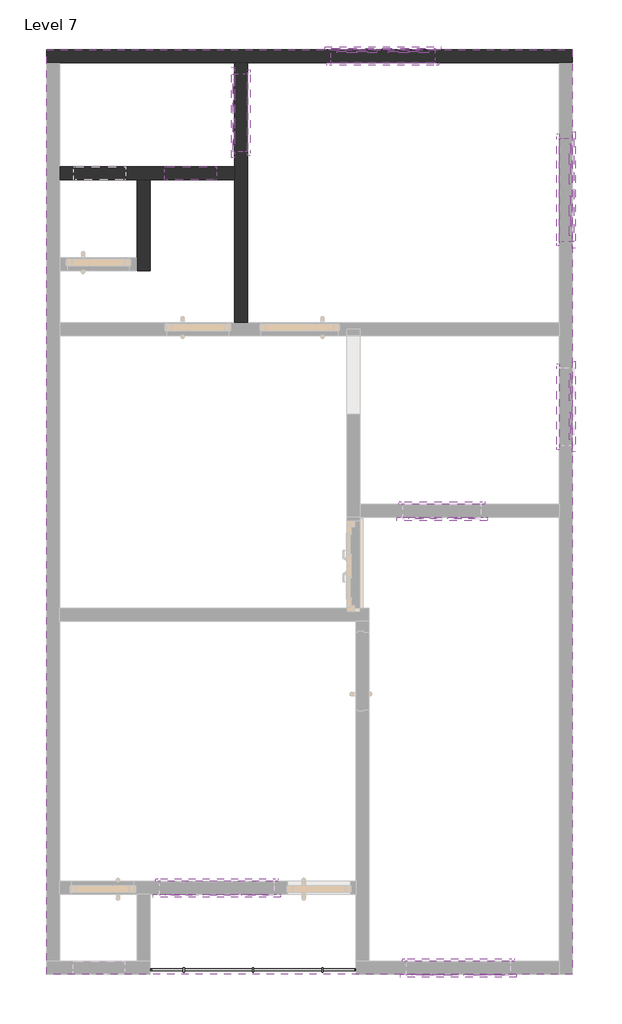
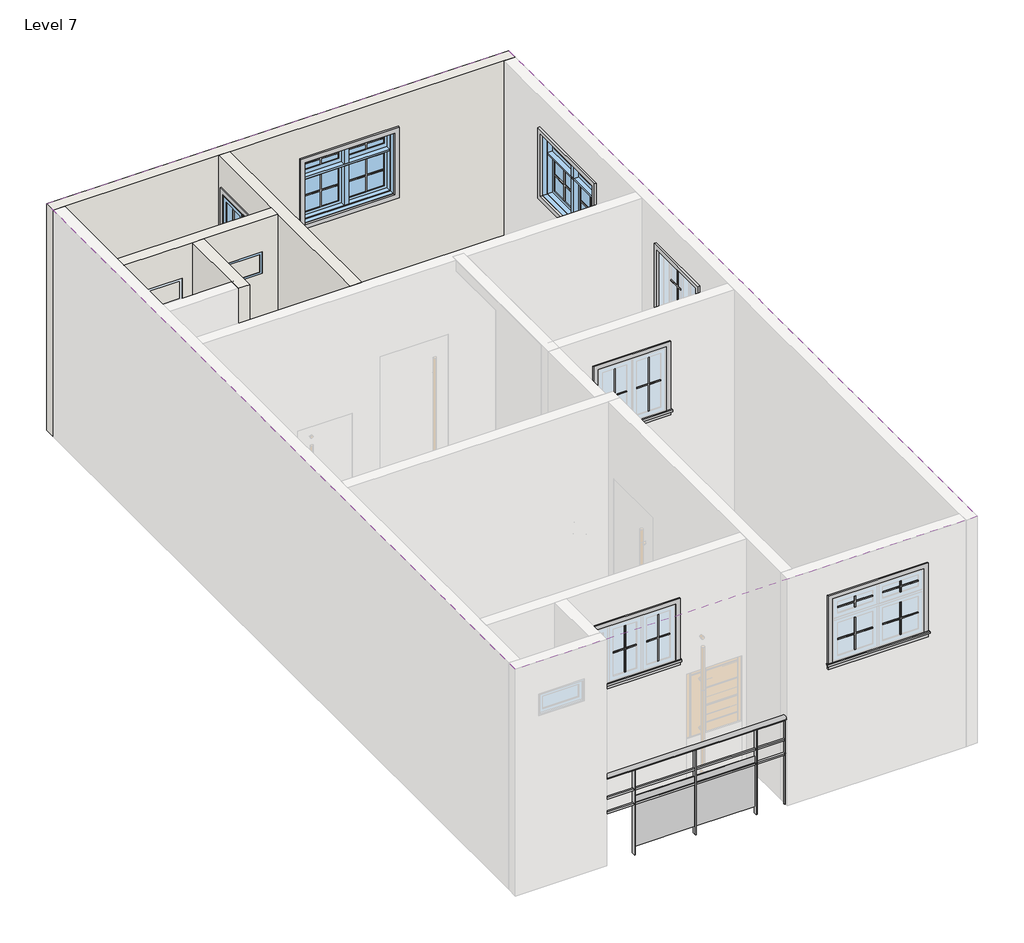
# One storey, part 2 of 2: 48 proxies, 7 walls, 5 windows, 1 covering, 1 railing.
"""IFC4 building model written with IfcOpenShell, lengths in millimetres."""

from ifc_helpers import new_model, si_unit, point, frame, origin, place, context, project, spatial, polyline, ellipse_curve, trimmed, outline, extrude, faceted_brep, transform, mapped, element, save
from ifc_brep_helpers import plane_surface, extruded_surface, advanced_brep
from components import m_muntin_pattern_2x2_m_muntin_pattern_2x2_ec2ff75e, m_muntin_pattern_2x2_m_muntin_pattern_2x2_6a19bea2, m_muntin_pattern_2x2_m_muntin_pattern_2x2_383df7b3, m_muntin_pattern_2x2_m_muntin_pattern_2x2_55460d9e, m_muntin_pattern_2x2_m_muntin_pattern_2x2_a9b7b7a9, m_muntin_pattern_2x2_m_muntin_pattern_2x2_c959817e, m_muntin_pattern_2x2_m_muntin_pattern_2x2_9259c5e2, m_trim_window_exterior_flat_with_sill_b1b88069, m_trim_window_exterior_flat_with_sill_8fa486dc, m_trim_window_exterior_flat_with_sill_2a9c44ae, m_trim_window_interior_flat_picture_frame_7d12f20c, m_trim_window_interior_flat_picture_frame_b6dd03a6, m_trim_window_interior_flat_picture_frame_c139440e, fixed_2_65c13adb, m_window_casement_double_3_e0bd8fa3, m_window_casement_double_awning_double_4_7efa9bbd

model = new_model("IFC4")

# Units and contexts
model_context = context("Model", 3, world=origin())
ifc_project = project(units=[si_unit("LENGTHUNIT", "METRE", prefix="MILLI")], contexts=[model_context])

# Site, building, storey
site = spatial("IfcSite", under=ifc_project)
building = spatial("IfcBuilding", under=site)
storey = spatial("IfcBuildingStorey", under=building, Name="Level 7", Elevation=10210.8)

# Proxies
placement = place(None, origin())
m_muntin_pattern_2x2_m_muntin_pattern_2x2_shape = m_muntin_pattern_2x2_m_muntin_pattern_2x2_ec2ff75e(model_context)
element("IfcBuildingElementProxy", 1, Name="M_Muntin Pattern_2x2 : M_Muntin Pattern_2x2", ObjectType="M_Muntin Pattern_2x2 : M_Muntin Pattern_2x2", at=placement, inside=storey, context=model_context, shape_type="MappedRepresentation", body=[
    mapped(m_muntin_pattern_2x2_m_muntin_pattern_2x2_shape, transform((-20164.8088079, 6316.5492053, 12109.45), x_axis=(1.0, 0.0, 0.0), y_axis=(0.0, 1.0, 0.0), z_axis=(0.0, 0.0, 1.0))),
])
element("IfcBuildingElementProxy", 2, Name="M_Muntin Pattern_2x2 : M_Muntin Pattern_2x2", ObjectType="M_Muntin Pattern_2x2 : M_Muntin Pattern_2x2", at=placement, inside=storey, context=model_context, shape_type="MappedRepresentation", body=[
    mapped(m_muntin_pattern_2x2_m_muntin_pattern_2x2_shape, transform((-17648.6213079, 4984.6367053, 12109.45), x_axis=(0.0, -1.0, 0.0), y_axis=(1.0, 0.0, 0.0), z_axis=(0.0, 0.0, 1.0))),
])
element("IfcBuildingElementProxy", 3, Name="M_Muntin Pattern_2x2 : M_Muntin Pattern_2x2", ObjectType="M_Muntin Pattern_2x2 : M_Muntin Pattern_2x2", at=placement, inside=storey, context=model_context, shape_type="MappedRepresentation", body=[
    mapped(m_muntin_pattern_2x2_m_muntin_pattern_2x2_shape, transform((-18672.7572454, -4510.2007947, 12109.45), x_axis=(-1.0, 0.0, 0.0), y_axis=(0.0, -1.0, 0.0), z_axis=(0.0, 0.0, 1.0))),
])
m_muntin_pattern_2x2_m_muntin_pattern_2x2_2_shape = m_muntin_pattern_2x2_m_muntin_pattern_2x2_6a19bea2(model_context)
element("IfcBuildingElementProxy", 4, Name="M_Muntin Pattern_2x2 : M_Muntin Pattern_2x2", ObjectType="M_Muntin Pattern_2x2 : M_Muntin Pattern_2x2", at=placement, inside=storey, context=model_context, shape_type="MappedRepresentation", body=[
    mapped(m_muntin_pattern_2x2_m_muntin_pattern_2x2_2_shape, transform((-19558.3838079, 6316.5492053, 12109.45), x_axis=(-1.0, 0.0, 0.0), y_axis=(0.0, -1.0, 0.0), z_axis=(0.0, 0.0, 1.0))),
])
element("IfcBuildingElementProxy", 5, Name="M_Muntin Pattern_2x2 : M_Muntin Pattern_2x2", ObjectType="M_Muntin Pattern_2x2 : M_Muntin Pattern_2x2", at=placement, inside=storey, context=model_context, shape_type="MappedRepresentation", body=[
    mapped(m_muntin_pattern_2x2_m_muntin_pattern_2x2_2_shape, transform((-17648.6213079, 4378.2117053, 12109.45), x_axis=(0.0, 1.0, 0.0), y_axis=(-1.0, 0.0, 0.0), z_axis=(0.0, 0.0, 1.0))),
])
element("IfcBuildingElementProxy", 6, Name="M_Muntin Pattern_2x2 : M_Muntin Pattern_2x2", ObjectType="M_Muntin Pattern_2x2 : M_Muntin Pattern_2x2", at=placement, inside=storey, context=model_context, shape_type="MappedRepresentation", body=[
    mapped(m_muntin_pattern_2x2_m_muntin_pattern_2x2_2_shape, transform((-19279.1822454, -4510.2007947, 12109.45), x_axis=(1.0, 0.0, 0.0), y_axis=(0.0, 1.0, 0.0), z_axis=(0.0, 0.0, 1.0))),
])
m_muntin_pattern_2x2_m_muntin_pattern_2x2_3_shape = m_muntin_pattern_2x2_m_muntin_pattern_2x2_383df7b3(model_context)
element("IfcBuildingElementProxy", 7, Name="M_Muntin Pattern_2x2 : M_Muntin Pattern_2x2", ObjectType="M_Muntin Pattern_2x2 : M_Muntin Pattern_2x2", at=placement, inside=storey, context=model_context, shape_type="MappedRepresentation", body=[
    mapped(m_muntin_pattern_2x2_m_muntin_pattern_2x2_3_shape, transform((-19558.3838079, 6316.5492053, 12709.45), x_axis=(-1.0, 0.0, 0.0), y_axis=(0.0, -1.0, 0.0), z_axis=(0.0, 0.0, 1.0))),
])
element("IfcBuildingElementProxy", 8, Name="M_Muntin Pattern_2x2 : M_Muntin Pattern_2x2", ObjectType="M_Muntin Pattern_2x2 : M_Muntin Pattern_2x2", at=placement, inside=storey, context=model_context, shape_type="MappedRepresentation", body=[
    mapped(m_muntin_pattern_2x2_m_muntin_pattern_2x2_3_shape, transform((-20164.8088079, 6316.5492053, 12709.45), x_axis=(-1.0, 0.0, 0.0), y_axis=(0.0, -1.0, 0.0), z_axis=(0.0, 0.0, 1.0))),
])
element("IfcBuildingElementProxy", 9, Name="M_Muntin Pattern_2x2 : M_Muntin Pattern_2x2", ObjectType="M_Muntin Pattern_2x2 : M_Muntin Pattern_2x2", at=placement, inside=storey, context=model_context, shape_type="MappedRepresentation", body=[
    mapped(m_muntin_pattern_2x2_m_muntin_pattern_2x2_3_shape, transform((-17648.6213079, 4378.2117053, 12709.45), x_axis=(0.0, 1.0, 0.0), y_axis=(-1.0, 0.0, 0.0), z_axis=(0.0, 0.0, 1.0))),
])
element("IfcBuildingElementProxy", 10, Name="M_Muntin Pattern_2x2 : M_Muntin Pattern_2x2", ObjectType="M_Muntin Pattern_2x2 : M_Muntin Pattern_2x2", at=placement, inside=storey, context=model_context, shape_type="MappedRepresentation", body=[
    mapped(m_muntin_pattern_2x2_m_muntin_pattern_2x2_3_shape, transform((-17648.6213079, 4984.6367053, 12709.45), x_axis=(0.0, 1.0, 0.0), y_axis=(-1.0, 0.0, 0.0), z_axis=(0.0, 0.0, 1.0))),
])
element("IfcBuildingElementProxy", 11, Name="M_Muntin Pattern_2x2 : M_Muntin Pattern_2x2", ObjectType="M_Muntin Pattern_2x2 : M_Muntin Pattern_2x2", at=placement, inside=storey, context=model_context, shape_type="MappedRepresentation", body=[
    mapped(m_muntin_pattern_2x2_m_muntin_pattern_2x2_3_shape, transform((-19279.1822454, -4510.2007947, 12709.45), x_axis=(1.0, 0.0, 0.0), y_axis=(0.0, 1.0, 0.0), z_axis=(0.0, 0.0, 1.0))),
])
element("IfcBuildingElementProxy", 12, Name="M_Muntin Pattern_2x2 : M_Muntin Pattern_2x2", ObjectType="M_Muntin Pattern_2x2 : M_Muntin Pattern_2x2", at=placement, inside=storey, context=model_context, shape_type="MappedRepresentation", body=[
    mapped(m_muntin_pattern_2x2_m_muntin_pattern_2x2_3_shape, transform((-18672.7572454, -4510.2007947, 12709.45), x_axis=(1.0, 0.0, 0.0), y_axis=(0.0, 1.0, 0.0), z_axis=(0.0, 0.0, 1.0))),
])
m_muntin_pattern_2x2_m_muntin_pattern_2x2_4_shape = m_muntin_pattern_2x2_m_muntin_pattern_2x2_55460d9e(model_context)
element("IfcBuildingElementProxy", 13, Name="M_Muntin Pattern_2x2 : M_Muntin Pattern_2x2", ObjectType="M_Muntin Pattern_2x2 : M_Muntin Pattern_2x2", at=placement, inside=storey, context=model_context, shape_type="MappedRepresentation", body=[
    mapped(m_muntin_pattern_2x2_m_muntin_pattern_2x2_4_shape, transform((-18939.9533391, 849.1992053, 12109.45), x_axis=(-1.0, 0.0, 0.0), y_axis=(0.0, -1.0, 0.0), z_axis=(0.0, 0.0, 1.0))),
])
element("IfcBuildingElementProxy", 14, Name="M_Muntin Pattern_2x2 : M_Muntin Pattern_2x2", ObjectType="M_Muntin Pattern_2x2 : M_Muntin Pattern_2x2", at=placement, inside=storey, context=model_context, shape_type="MappedRepresentation", body=[
    mapped(m_muntin_pattern_2x2_m_muntin_pattern_2x2_4_shape, transform((-17648.6213079, 2366.8492053, 12109.45), x_axis=(0.0, -1.0, 0.0), y_axis=(1.0, 0.0, 0.0), z_axis=(0.0, 0.0, 1.0))),
])
element("IfcBuildingElementProxy", 15, Name="M_Muntin Pattern_2x2 : M_Muntin Pattern_2x2", ObjectType="M_Muntin Pattern_2x2 : M_Muntin Pattern_2x2", at=placement, inside=storey, context=model_context, shape_type="MappedRepresentation", body=[
    mapped(m_muntin_pattern_2x2_m_muntin_pattern_2x2_4_shape, transform((-21591.9713079, 5362.4617053, 12109.45), x_axis=(0.0, 1.0, 0.0), y_axis=(-1.0, 0.0, 0.0), z_axis=(0.0, 0.0, 1.0))),
])
element("IfcBuildingElementProxy", 16, Name="M_Muntin Pattern_2x2 : M_Muntin Pattern_2x2", ObjectType="M_Muntin Pattern_2x2 : M_Muntin Pattern_2x2", at=placement, inside=storey, context=model_context, shape_type="MappedRepresentation", body=[
    mapped(m_muntin_pattern_2x2_m_muntin_pattern_2x2_4_shape, transform((-18939.9533391, 849.1992053, 12109.45), x_axis=(-1.0, 0.0, 0.0), y_axis=(0.0, -1.0, 0.0), z_axis=(0.0, 0.0, 1.0))),
])
element("IfcBuildingElementProxy", 17, Name="M_Muntin Pattern_2x2 : M_Muntin Pattern_2x2", ObjectType="M_Muntin Pattern_2x2 : M_Muntin Pattern_2x2", at=placement, inside=storey, context=model_context, shape_type="MappedRepresentation", body=[
    mapped(m_muntin_pattern_2x2_m_muntin_pattern_2x2_4_shape, transform((-21591.9713079, 5362.4617053, 12109.45), x_axis=(0.0, 1.0, 0.0), y_axis=(-1.0, 0.0, 0.0), z_axis=(0.0, 0.0, 1.0))),
])
m_muntin_pattern_2x2_m_muntin_pattern_2x2_5_shape = m_muntin_pattern_2x2_m_muntin_pattern_2x2_a9b7b7a9(model_context)
element("IfcBuildingElementProxy", 18, Name="M_Muntin Pattern_2x2 : M_Muntin Pattern_2x2", ObjectType="M_Muntin Pattern_2x2 : M_Muntin Pattern_2x2", at=placement, inside=storey, context=model_context, shape_type="MappedRepresentation", body=[
    mapped(m_muntin_pattern_2x2_m_muntin_pattern_2x2_5_shape, transform((-19393.9783391, 849.1992053, 12109.45), x_axis=(1.0, 0.0, 0.0), y_axis=(0.0, 1.0, 0.0), z_axis=(0.0, 0.0, 1.0))),
])
element("IfcBuildingElementProxy", 19, Name="M_Muntin Pattern_2x2 : M_Muntin Pattern_2x2", ObjectType="M_Muntin Pattern_2x2 : M_Muntin Pattern_2x2", at=placement, inside=storey, context=model_context, shape_type="MappedRepresentation", body=[
    mapped(m_muntin_pattern_2x2_m_muntin_pattern_2x2_5_shape, transform((-17648.6213079, 1912.8242053, 12109.45), x_axis=(0.0, 1.0, 0.0), y_axis=(-1.0, 0.0, 0.0), z_axis=(0.0, 0.0, 1.0))),
])
element("IfcBuildingElementProxy", 20, Name="M_Muntin Pattern_2x2 : M_Muntin Pattern_2x2", ObjectType="M_Muntin Pattern_2x2 : M_Muntin Pattern_2x2", at=placement, inside=storey, context=model_context, shape_type="MappedRepresentation", body=[
    mapped(m_muntin_pattern_2x2_m_muntin_pattern_2x2_5_shape, transform((-21591.9713079, 5816.4867053, 12109.45), x_axis=(0.0, -1.0, 0.0), y_axis=(1.0, 0.0, 0.0), z_axis=(0.0, 0.0, 1.0))),
])
element("IfcBuildingElementProxy", 21, Name="M_Muntin Pattern_2x2 : M_Muntin Pattern_2x2", ObjectType="M_Muntin Pattern_2x2 : M_Muntin Pattern_2x2", at=placement, inside=storey, context=model_context, shape_type="MappedRepresentation", body=[
    mapped(m_muntin_pattern_2x2_m_muntin_pattern_2x2_5_shape, transform((-19393.9783391, 849.1992053, 12109.45), x_axis=(1.0, 0.0, 0.0), y_axis=(0.0, 1.0, 0.0), z_axis=(0.0, 0.0, 1.0))),
])
element("IfcBuildingElementProxy", 22, Name="M_Muntin Pattern_2x2 : M_Muntin Pattern_2x2", ObjectType="M_Muntin Pattern_2x2 : M_Muntin Pattern_2x2", at=placement, inside=storey, context=model_context, shape_type="MappedRepresentation", body=[
    mapped(m_muntin_pattern_2x2_m_muntin_pattern_2x2_5_shape, transform((-21591.9713079, 5816.4867053, 12109.45), x_axis=(0.0, -1.0, 0.0), y_axis=(1.0, 0.0, 0.0), z_axis=(0.0, 0.0, 1.0))),
])
m_muntin_pattern_2x2_m_muntin_pattern_2x2_6_shape = m_muntin_pattern_2x2_m_muntin_pattern_2x2_c959817e(model_context)
element("IfcBuildingElementProxy", 23, Name="M_Muntin Pattern_2x2 : M_Muntin Pattern_2x2", ObjectType="M_Muntin Pattern_2x2 : M_Muntin Pattern_2x2", at=placement, inside=storey, context=model_context, shape_type="MappedRepresentation", body=[
    mapped(m_muntin_pattern_2x2_m_muntin_pattern_2x2_6_shape, transform((-21364.4296412, -3570.4007947, 12109.45), x_axis=(-1.0, 0.0, 0.0), y_axis=(0.0, -1.0, 0.0), z_axis=(0.0, 0.0, 1.0))),
])
element("IfcBuildingElementProxy", 24, Name="M_Muntin Pattern_2x2 : M_Muntin Pattern_2x2", ObjectType="M_Muntin Pattern_2x2 : M_Muntin Pattern_2x2", at=placement, inside=storey, context=model_context, shape_type="MappedRepresentation", body=[
    mapped(m_muntin_pattern_2x2_m_muntin_pattern_2x2_6_shape, transform((-21364.4296412, -3570.4007947, 12109.45), x_axis=(-1.0, 0.0, 0.0), y_axis=(0.0, -1.0, 0.0), z_axis=(0.0, 0.0, 1.0))),
])
m_muntin_pattern_2x2_m_muntin_pattern_2x2_7_shape = m_muntin_pattern_2x2_m_muntin_pattern_2x2_9259c5e2(model_context)
element("IfcBuildingElementProxy", 25, Name="M_Muntin Pattern_2x2 : M_Muntin Pattern_2x2", ObjectType="M_Muntin Pattern_2x2 : M_Muntin Pattern_2x2", at=placement, inside=storey, context=model_context, shape_type="MappedRepresentation", body=[
    mapped(m_muntin_pattern_2x2_m_muntin_pattern_2x2_7_shape, transform((-22257.6629746, -3570.4007947, 12109.45), x_axis=(1.0, 0.0, 0.0), y_axis=(0.0, 1.0, 0.0), z_axis=(0.0, 0.0, 1.0))),
])
element("IfcBuildingElementProxy", 26, Name="M_Muntin Pattern_2x2 : M_Muntin Pattern_2x2", ObjectType="M_Muntin Pattern_2x2 : M_Muntin Pattern_2x2", at=placement, inside=storey, context=model_context, shape_type="MappedRepresentation", body=[
    mapped(m_muntin_pattern_2x2_m_muntin_pattern_2x2_7_shape, transform((-21811.0463079, -3570.4007947, 12109.45), x_axis=(1.0, 0.0, 0.0), y_axis=(0.0, 1.0, 0.0), z_axis=(0.0, 0.0, 1.0))),
])
element("IfcBuildingElementProxy", 27, Name="M_Muntin Pattern_2x2 : M_Muntin Pattern_2x2", ObjectType="M_Muntin Pattern_2x2 : M_Muntin Pattern_2x2", at=placement, inside=storey, context=model_context, shape_type="MappedRepresentation", body=[
    mapped(m_muntin_pattern_2x2_m_muntin_pattern_2x2_7_shape, transform((-22257.6629746, -3570.4007947, 12109.45), x_axis=(1.0, 0.0, 0.0), y_axis=(0.0, 1.0, 0.0), z_axis=(0.0, 0.0, 1.0))),
])
element("IfcBuildingElementProxy", 28, Name="M_Muntin Pattern_2x2 : M_Muntin Pattern_2x2", ObjectType="M_Muntin Pattern_2x2 : M_Muntin Pattern_2x2", at=placement, inside=storey, context=model_context, shape_type="MappedRepresentation", body=[
    mapped(m_muntin_pattern_2x2_m_muntin_pattern_2x2_7_shape, transform((-21811.0463079, -3570.4007947, 12109.45), x_axis=(1.0, 0.0, 0.0), y_axis=(0.0, 1.0, 0.0), z_axis=(0.0, 0.0, 1.0))),
])
m_trim_window_exterior_flat_with_sill_shape = m_trim_window_exterior_flat_with_sill_b1b88069(model_context)
element("IfcBuildingElementProxy", 29, Name="M_Trim-Window-Exterior-Flat : with Sill", ObjectType="M_Trim-Window-Exterior-Flat : with Sill", at=placement, inside=storey, context=model_context, shape_type="MappedRepresentation", body=[
    mapped(m_trim_window_exterior_flat_with_sill_shape, transform((-19861.5963079, 6326.0742053, 12939.6), x_axis=(-1.0, 0.0, 0.0), y_axis=(0.0, 0.0, 1.0), z_axis=(0.0, 1.0, 0.0))),
])
element("IfcBuildingElementProxy", 30, Name="M_Trim-Window-Exterior-Flat : with Sill", ObjectType="M_Trim-Window-Exterior-Flat : with Sill", at=placement, inside=storey, context=model_context, shape_type="MappedRepresentation", body=[
    mapped(m_trim_window_exterior_flat_with_sill_shape, transform((-17639.0963079, 4681.4242053, 12939.6), x_axis=(0.0, 1.0, 0.0), y_axis=(0.0, 0.0, 1.0), z_axis=(1.0, 0.0, 0.0))),
])
element("IfcBuildingElementProxy", 31, Name="M_Trim-Window-Exterior-Flat : with Sill", ObjectType="M_Trim-Window-Exterior-Flat : with Sill", at=placement, inside=storey, context=model_context, shape_type="MappedRepresentation", body=[
    mapped(m_trim_window_exterior_flat_with_sill_shape, transform((-18975.9697454, -4519.7257947, 12939.6), x_axis=(1.0, 0.0, 0.0), y_axis=(0.0, 0.0, 1.0), z_axis=(0.0, -1.0, 0.0))),
])
m_trim_window_exterior_flat_with_sill_2_shape = m_trim_window_exterior_flat_with_sill_8fa486dc(model_context)
element("IfcBuildingElementProxy", 32, Name="M_Trim-Window-Exterior-Flat : with Sill", ObjectType="M_Trim-Window-Exterior-Flat : with Sill", at=placement, inside=storey, context=model_context, shape_type="MappedRepresentation", body=[
    mapped(m_trim_window_exterior_flat_with_sill_2_shape, transform((-19166.9658391, 839.6742053, 12939.6), x_axis=(1.0, 0.0, 0.0), y_axis=(0.0, 0.0, 1.0), z_axis=(0.0, -1.0, 0.0))),
])
element("IfcBuildingElementProxy", 33, Name="M_Trim-Window-Exterior-Flat : with Sill", ObjectType="M_Trim-Window-Exterior-Flat : with Sill", at=placement, inside=storey, context=model_context, shape_type="MappedRepresentation", body=[
    mapped(m_trim_window_exterior_flat_with_sill_2_shape, transform((-17639.0963079, 2139.8367053, 12939.6), x_axis=(0.0, 1.0, 0.0), y_axis=(0.0, 0.0, 1.0), z_axis=(1.0, 0.0, 0.0))),
])
element("IfcBuildingElementProxy", 34, Name="M_Trim-Window-Exterior-Flat : with Sill", ObjectType="M_Trim-Window-Exterior-Flat : with Sill", at=placement, inside=storey, context=model_context, shape_type="MappedRepresentation", body=[
    mapped(m_trim_window_exterior_flat_with_sill_2_shape, transform((-21601.4963079, 5589.4742053, 12939.6), x_axis=(0.0, -1.0, 0.0), y_axis=(0.0, 0.0, 1.0), z_axis=(-1.0, 0.0, 0.0))),
])
element("IfcBuildingElementProxy", 35, Name="M_Trim-Window-Exterior-Flat : with Sill", ObjectType="M_Trim-Window-Exterior-Flat : with Sill", at=placement, inside=storey, context=model_context, shape_type="MappedRepresentation", body=[
    mapped(m_trim_window_exterior_flat_with_sill_2_shape, transform((-19166.9658391, 839.6742053, 12939.6), x_axis=(1.0, 0.0, 0.0), y_axis=(0.0, 0.0, 1.0), z_axis=(0.0, -1.0, 0.0))),
])
element("IfcBuildingElementProxy", 36, Name="M_Trim-Window-Exterior-Flat : with Sill", ObjectType="M_Trim-Window-Exterior-Flat : with Sill", at=placement, inside=storey, context=model_context, shape_type="MappedRepresentation", body=[
    mapped(m_trim_window_exterior_flat_with_sill_2_shape, transform((-21601.4963079, 5589.4742053, 12939.6), x_axis=(0.0, -1.0, 0.0), y_axis=(0.0, 0.0, 1.0), z_axis=(-1.0, 0.0, 0.0))),
])
m_trim_window_exterior_flat_with_sill_3_shape = m_trim_window_exterior_flat_with_sill_2a9c44ae(model_context)
element("IfcBuildingElementProxy", 37, Name="M_Trim-Window-Exterior-Flat : with Sill", ObjectType="M_Trim-Window-Exterior-Flat : with Sill", at=placement, inside=storey, context=model_context, shape_type="MappedRepresentation", body=[
    mapped(m_trim_window_exterior_flat_with_sill_3_shape, transform((-21811.0463079, -3579.9257947, 12839.6), x_axis=(1.0, 0.0, 0.0), y_axis=(0.0, 0.0, 1.0), z_axis=(0.0, -1.0, 0.0))),
])
element("IfcBuildingElementProxy", 38, Name="M_Trim-Window-Exterior-Flat : with Sill", ObjectType="M_Trim-Window-Exterior-Flat : with Sill", at=placement, inside=storey, context=model_context, shape_type="MappedRepresentation", body=[
    mapped(m_trim_window_exterior_flat_with_sill_3_shape, transform((-21811.0463079, -3579.9257947, 12839.6), x_axis=(1.0, 0.0, 0.0), y_axis=(0.0, 0.0, 1.0), z_axis=(0.0, -1.0, 0.0))),
])
m_trim_window_interior_flat_picture_frame_shape = m_trim_window_interior_flat_picture_frame_7d12f20c(model_context)
element("IfcBuildingElementProxy", 39, Name="M_Trim-Window-Interior-Flat : Picture Frame", ObjectType="M_Trim-Window-Interior-Flat : Picture Frame", at=placement, inside=storey, context=model_context, shape_type="MappedRepresentation", body=[
    mapped(m_trim_window_interior_flat_picture_frame_shape, transform((-19861.5963079, 6173.6742053, 12939.6), x_axis=(1.0, 0.0, 0.0), y_axis=(0.0, 0.0, 1.0), z_axis=(0.0, -1.0, 0.0))),
])
element("IfcBuildingElementProxy", 40, Name="M_Trim-Window-Interior-Flat : Picture Frame", ObjectType="M_Trim-Window-Interior-Flat : Picture Frame", at=placement, inside=storey, context=model_context, shape_type="MappedRepresentation", body=[
    mapped(m_trim_window_interior_flat_picture_frame_shape, transform((-17791.4963079, 4681.4242053, 12939.6), x_axis=(0.0, -1.0, 0.0), y_axis=(0.0, 0.0, 1.0), z_axis=(-1.0, 0.0, 0.0))),
])
element("IfcBuildingElementProxy", 41, Name="M_Trim-Window-Interior-Flat : Picture Frame", ObjectType="M_Trim-Window-Interior-Flat : Picture Frame", at=placement, inside=storey, context=model_context, shape_type="MappedRepresentation", body=[
    mapped(m_trim_window_interior_flat_picture_frame_shape, transform((-18975.9697454, -4367.3257947, 12939.6), x_axis=(-1.0, 0.0, 0.0), y_axis=(0.0, 0.0, 1.0), z_axis=(0.0, 1.0, 0.0))),
])
m_trim_window_interior_flat_picture_frame_2_shape = m_trim_window_interior_flat_picture_frame_b6dd03a6(model_context)
element("IfcBuildingElementProxy", 42, Name="M_Trim-Window-Interior-Flat : Picture Frame", ObjectType="M_Trim-Window-Interior-Flat : Picture Frame", at=placement, inside=storey, context=model_context, shape_type="MappedRepresentation", body=[
    mapped(m_trim_window_interior_flat_picture_frame_2_shape, transform((-19166.9658391, 992.0742053, 12939.6), x_axis=(-1.0, 0.0, 0.0), y_axis=(0.0, 0.0, 1.0), z_axis=(0.0, 1.0, 0.0))),
])
element("IfcBuildingElementProxy", 43, Name="M_Trim-Window-Interior-Flat : Picture Frame", ObjectType="M_Trim-Window-Interior-Flat : Picture Frame", at=placement, inside=storey, context=model_context, shape_type="MappedRepresentation", body=[
    mapped(m_trim_window_interior_flat_picture_frame_2_shape, transform((-17791.4963079, 2139.8367053, 12939.6), x_axis=(0.0, -1.0, 0.0), y_axis=(0.0, 0.0, 1.0), z_axis=(-1.0, 0.0, 0.0))),
])
element("IfcBuildingElementProxy", 44, Name="M_Trim-Window-Interior-Flat : Picture Frame", ObjectType="M_Trim-Window-Interior-Flat : Picture Frame", at=placement, inside=storey, context=model_context, shape_type="MappedRepresentation", body=[
    mapped(m_trim_window_interior_flat_picture_frame_2_shape, transform((-21449.0963079, 5589.4742053, 12939.6), x_axis=(0.0, 1.0, 0.0), y_axis=(0.0, 0.0, 1.0), z_axis=(1.0, 0.0, 0.0))),
])
element("IfcBuildingElementProxy", 45, Name="M_Trim-Window-Interior-Flat : Picture Frame", ObjectType="M_Trim-Window-Interior-Flat : Picture Frame", at=placement, inside=storey, context=model_context, shape_type="MappedRepresentation", body=[
    mapped(m_trim_window_interior_flat_picture_frame_2_shape, transform((-19166.9658391, 992.0742053, 12939.6), x_axis=(-1.0, 0.0, 0.0), y_axis=(0.0, 0.0, 1.0), z_axis=(0.0, 1.0, 0.0))),
])
element("IfcBuildingElementProxy", 46, Name="M_Trim-Window-Interior-Flat : Picture Frame", ObjectType="M_Trim-Window-Interior-Flat : Picture Frame", at=placement, inside=storey, context=model_context, shape_type="MappedRepresentation", body=[
    mapped(m_trim_window_interior_flat_picture_frame_2_shape, transform((-21449.0963079, 5589.4742053, 12939.6), x_axis=(0.0, 1.0, 0.0), y_axis=(0.0, 0.0, 1.0), z_axis=(1.0, 0.0, 0.0))),
])
m_trim_window_interior_flat_picture_frame_3_shape = m_trim_window_interior_flat_picture_frame_c139440e(model_context)
element("IfcBuildingElementProxy", 47, Name="M_Trim-Window-Interior-Flat : Picture Frame", ObjectType="M_Trim-Window-Interior-Flat : Picture Frame", at=placement, inside=storey, context=model_context, shape_type="MappedRepresentation", body=[
    mapped(m_trim_window_interior_flat_picture_frame_3_shape, transform((-21811.0463079, -3427.5257947, 12839.6), x_axis=(-1.0, 0.0, 0.0), y_axis=(0.0, 0.0, 1.0), z_axis=(0.0, 1.0, 0.0))),
])
element("IfcBuildingElementProxy", 48, Name="M_Trim-Window-Interior-Flat : Picture Frame", ObjectType="M_Trim-Window-Interior-Flat : Picture Frame", at=placement, inside=storey, context=model_context, shape_type="MappedRepresentation", body=[
    mapped(m_trim_window_interior_flat_picture_frame_3_shape, transform((-21811.0463079, -3427.5257947, 12839.6), x_axis=(-1.0, 0.0, 0.0), y_axis=(0.0, 0.0, 1.0), z_axis=(0.0, 1.0, 0.0))),
])

# Covering
element("IfcCovering", 49, ObjectType="2' x 4' ACT System", at=placement, inside=storey, context=model_context, shape_type="SweptSolid", body=[
    extrude(outline(polyline([(-23811.2963079, -4519.7257947), (-23811.2963079, 6326.0742053), (-17639.0963079, 6326.0742053), (-17639.0963079, -4519.7257947), (-22309.2664727, -4519.7257947), (-23811.2963079, -4519.7257947)])), frame((0.0, 0.0, 13411.2), z_axis=(0.0, 0.0, 1.0), x_axis=(1.0, 0.0, 0.0)), (0.0, 0.0, 1.0), 57.15),
])

# Railing
element("IfcRailing", 50, ObjectType="Glass Panel - Bottom Fill", at=placement, inside=storey, context=model_context, shape_type="SolidModel", body=[
    advanced_brep(
    [(-22592.0963079, -4430.8257947, 11430.0), (-22592.0963079, -4507.0257947, 11430.0), (-20179.0963079, -4430.8257947, 11430.0), (-20179.0963079, -4507.0257947, 11430.0)],
    [
        (0, 1, ellipse_curve(frame((-22592.0963079, -4468.9257947, 11430.0), z_axis=(-1.0, 0.0, 0.0), x_axis=(0.0, -1.0, 0.0)), 38.1, 28.575)),
        (1, 0, ellipse_curve(frame((-22592.0963079, -4468.9257947, 11430.0), z_axis=(-1.0, 0.0, 0.0), x_axis=(0.0, -1.0, 0.0)), 38.1, 28.575)),
        (2, 3, ellipse_curve(frame((-20179.0963079, -4468.9257947, 11430.0), z_axis=(1.0, 0.0, 0.0), x_axis=(0.0, -1.0, 0.0)), 38.1, 28.575)),
        (3, 2, ellipse_curve(frame((-20179.0963079, -4468.9257947, 11430.0), z_axis=(1.0, 0.0, 0.0), x_axis=(0.0, -1.0, 0.0)), 38.1, 28.575)),
        (0, 2),
        (3, 1),
    ],
    [
        plane_surface(frame((-22592.0963079, -4468.9257947, 11430.0), z_axis=(-1.0, 0.0, 0.0), x_axis=(0.0, 1.0, 0.0))),
        plane_surface(frame((-20179.0963079, -4468.9257947, 11430.0), z_axis=(1.0, 0.0, 0.0), x_axis=(0.0, 1.0, 0.0))),
        extruded_surface(trimmed(ellipse_curve(frame((-20179.0963079, -4468.9257947, 11430.0), z_axis=(-1.0, 0.0, 0.0), x_axis=(0.0, -1.0, 0.0)), 38.1, 28.575), [point((-20179.0963079, -4430.8257947, 11430.0))], [point((-20179.0963079, -4507.0257947, 11430.0))], True, "CARTESIAN"), (-2413.0, 0.0, 0.0), 2413.0),
        extruded_surface(trimmed(ellipse_curve(frame((-20179.0963079, -4468.9257947, 11430.0), z_axis=(-1.0, 0.0, 0.0), x_axis=(0.0, -1.0, 0.0)), 38.1, 28.575), [point((-20179.0963079, -4507.0257947, 11430.0))], [point((-20179.0963079, -4430.8257947, 11430.0))], True, "CARTESIAN"), (-2413.0, 0.0, 0.0), 2413.0),
    ],
    [
        (0, [[1, 2]]),
        (1, [[3, 4]]),
        (2, [[-1, 5, -4, 6]]),
        (3, [[-2, -6, -3, -5]]),
    ],
),
    extrude(outline(polyline([(-22592.0963079, -4481.6257947), (-22592.0963079, -4456.2257947), (-20179.0963079, -4456.2257947), (-20179.0963079, -4481.6257947), (-22592.0963079, -4481.6257947)])), frame((0.0, 0.0, 11112.5), z_axis=(0.0, 0.0, 1.0), x_axis=(1.0, 0.0, 0.0)), (0.0, 0.0, 1.0), 25.4),
    extrude(outline(polyline([(-22592.0963079, -4481.6257947), (-22592.0963079, -4456.2257947), (-20179.0963079, -4456.2257947), (-20179.0963079, -4481.6257947), (-22592.0963079, -4481.6257947)])), frame((0.0, 0.0, 10909.3), z_axis=(0.0, 0.0, 1.0), x_axis=(1.0, 0.0, 0.0)), (0.0, 0.0, 1.0), 25.4),
    extrude(outline(polyline([(-20579.1463079, -4494.3257947), (-20579.1463079, -4443.5257947), (-20566.4463079, -4443.5257947), (-20566.4463079, -4494.3257947), (-20579.1463079, -4494.3257947)])), frame((0.0, 0.0, 10210.8), z_axis=(0.0, 0.0, 1.0), x_axis=(1.0, 0.0, 0.0)), (0.0, 0.0, 1.0), 1190.625),
    extrude(outline(polyline([(-21385.5963079, -4462.3906377), (-20572.7963079, -4462.3906377), (-20572.7963079, -4468.7406377), (-21385.5963079, -4468.7406377), (-21385.5963079, -4462.3906377)])), frame((0.0, 0.0, 10312.4), z_axis=(0.0, 0.0, 1.0), x_axis=(1.0, 0.0, 0.0)), (0.0, 0.0, 1.0), 711.2),
    extrude(outline(polyline([(-21391.9463079, -4494.3257947), (-21391.9463079, -4443.5257947), (-21379.2463079, -4443.5257947), (-21379.2463079, -4494.3257947), (-21391.9463079, -4494.3257947)])), frame((0.0, 0.0, 10210.8), z_axis=(0.0, 0.0, 1.0), x_axis=(1.0, 0.0, 0.0)), (0.0, 0.0, 1.0), 1190.625),
    extrude(outline(polyline([(-22198.3963079, -4462.3906377), (-21385.5963079, -4462.3906377), (-21385.5963079, -4468.7406377), (-22198.3963079, -4468.7406377), (-22198.3963079, -4462.3906377)])), frame((0.0, 0.0, 10312.4), z_axis=(0.0, 0.0, 1.0), x_axis=(1.0, 0.0, 0.0)), (0.0, 0.0, 1.0), 711.2),
    extrude(outline(polyline([(-22204.7463079, -4494.3257947), (-22204.7463079, -4443.5257947), (-22192.0463079, -4443.5257947), (-22192.0463079, -4494.3257947), (-22204.7463079, -4494.3257947)])), frame((0.0, 0.0, 10210.8), z_axis=(0.0, 0.0, 1.0), x_axis=(1.0, 0.0, 0.0)), (0.0, 0.0, 1.0), 1190.625),
    extrude(outline(polyline([(-20191.7963079, -4478.4507947), (-20191.7963079, -4459.4007947), (-20172.7463079, -4459.4007947), (-20172.7463079, -4478.4507947), (-20191.7963079, -4478.4507947)])), frame((0.0, 0.0, 10210.8), z_axis=(0.0, 0.0, 1.0), x_axis=(1.0, 0.0, 0.0)), (0.0, 0.0, 1.0), 1190.625),
    extrude(outline(polyline([(-22598.4463079, -4478.4507947), (-22598.4463079, -4459.4007947), (-22579.3963079, -4459.4007947), (-22579.3963079, -4478.4507947), (-22598.4463079, -4478.4507947)])), frame((0.0, 0.0, 10210.8), z_axis=(0.0, 0.0, 1.0), x_axis=(1.0, 0.0, 0.0)), (0.0, 0.0, 1.0), 1190.625),
])

# Walls
element("IfcWall", 51, ObjectType="Generic - 6\"", at=placement, inside=storey, context=model_context, shape_type="Brep", body=[
    faceted_brep([(-23811.2963079, 6173.6742053, 10210.8), (-23658.8963079, 6173.6742053, 10210.8), (-21601.4963079, 6173.6742053, 10210.8), (-21449.0963079, 6173.6742053, 10210.8), (-17791.4963079, 6173.6742053, 10210.8), (-17639.0963079, 6173.6742053, 10210.8), (-17639.0963079, 6173.6742053, 13411.2), (-17791.4963079, 6173.6742053, 13411.2), (-21449.0963079, 6173.6742053, 13411.2), (-21601.4963079, 6173.6742053, 13411.2), (-23658.8963079, 6173.6742053, 13411.2), (-23811.2963079, 6173.6742053, 13411.2), (-19251.9963079, 6173.6742053, 12939.6), (-19251.9963079, 6173.6742053, 12039.6), (-20471.1963079, 6173.6742053, 12039.6), (-20471.1963079, 6173.6742053, 12939.6), (-23811.2963079, 6326.0742053, 10210.8), (-23811.2963079, 6326.0742053, 13411.2), (-17639.0963079, 6326.0742053, 13411.2), (-17639.0963079, 6326.0742053, 10210.8), (-19251.9963079, 6326.0742053, 12939.6), (-20471.1963079, 6326.0742053, 12939.6), (-20471.1963079, 6326.0742053, 12039.6), (-19251.9963079, 6326.0742053, 12039.6)], [[[0, 1, 2, 3, 4, 5, 6, 7, 8, 9, 10, 11], [12, 13, 14, 15]], [[16, 17, 18, 19], [20, 21, 22, 23]], [[5, 4, 3, 2, 1, 0, 16, 19]], [[11, 10, 9, 8, 7, 6, 18, 17]], [[6, 5, 19, 18]], [[0, 11, 17, 16]], [[13, 12, 20, 23]], [[14, 13, 23, 22]], [[15, 14, 22, 21]], [[12, 15, 21, 20]]]),
])
element("IfcWall", 52, ObjectType="Generic - 6\"", at=placement, inside=storey, context=model_context, shape_type="Brep", body=[
    faceted_brep([(-21601.4963079, 6173.6742053, 10210.8), (-21601.4963079, 4954.4742053, 10210.8), (-21601.4963079, 4802.0742053, 10210.8), (-21601.4963079, 3125.6742053, 10210.8), (-21601.4963079, 3125.6742053, 13411.2), (-21601.4963079, 4802.0742053, 13411.2), (-21601.4963079, 4954.4742053, 13411.2), (-21601.4963079, 6173.6742053, 13411.2), (-21601.4963079, 6046.6742053, 12939.6), (-21601.4963079, 5132.2742053, 12939.6), (-21601.4963079, 5132.2742053, 12039.6), (-21601.4963079, 6046.6742053, 12039.6), (-21449.0963079, 6173.6742053, 10210.8), (-21449.0963079, 6173.6742053, 13411.2), (-21449.0963079, 3125.6742053, 13411.2), (-21449.0963079, 3125.6742053, 10210.8), (-21449.0963079, 6046.6742053, 12939.6), (-21449.0963079, 6046.6742053, 12039.6), (-21449.0963079, 5132.2742053, 12039.6), (-21449.0963079, 5132.2742053, 12939.6)], [[[0, 1, 2, 3, 4, 5, 6, 7], [8, 9, 10, 11]], [[12, 13, 14, 15], [16, 17, 18, 19]], [[3, 2, 1, 0, 12, 15]], [[7, 6, 5, 4, 14, 13]], [[0, 7, 13, 12]], [[4, 3, 15, 14]], [[17, 16, 8, 11]], [[18, 17, 11, 10]], [[19, 18, 10, 9]], [[16, 19, 9, 8]]]),
])
element("IfcWall", 53, ObjectType="Generic - 6\"", at=placement, inside=storey, context=model_context, shape_type="Brep", body=[
    faceted_brep([(-23658.8963079, 4802.0742053, 10210.8), (-22744.4963079, 4802.0742053, 10210.8), (-22592.0963079, 4802.0742053, 10210.8), (-21601.4963079, 4802.0742053, 10210.8), (-21601.4963079, 4802.0742053, 13411.2), (-22592.0963079, 4802.0742053, 13411.2), (-22744.4963079, 4802.0742053, 13411.2), (-23658.8963079, 4802.0742053, 13411.2), (-22880.5252141, 4802.0742053, 12954.0), (-22880.5252141, 4802.0742053, 12649.2), (-23490.1252141, 4802.0742053, 12649.2), (-23490.1252141, 4802.0742053, 12954.0), (-21812.6338079, 4802.0742053, 12954.0), (-21812.6338079, 4802.0742053, 12649.2), (-22422.2338079, 4802.0742053, 12649.2), (-22422.2338079, 4802.0742053, 12954.0), (-23658.8963079, 4954.4742053, 10210.8), (-23658.8963079, 4954.4742053, 13411.2), (-21601.4963079, 4954.4742053, 13411.2), (-21601.4963079, 4954.4742053, 10210.8), (-22880.5252141, 4954.4742053, 12954.0), (-23490.1252141, 4954.4742053, 12954.0), (-23490.1252141, 4954.4742053, 12649.2), (-22880.5252141, 4954.4742053, 12649.2), (-21812.6338079, 4954.4742053, 12954.0), (-22422.2338079, 4954.4742053, 12954.0), (-22422.2338079, 4954.4742053, 12649.2), (-21812.6338079, 4954.4742053, 12649.2)], [[[0, 1, 2, 3, 4, 5, 6, 7], [8, 9, 10, 11], [12, 13, 14, 15]], [[16, 17, 18, 19], [20, 21, 22, 23], [24, 25, 26, 27]], [[3, 2, 1, 0, 16, 19]], [[7, 6, 5, 4, 18, 17]], [[0, 7, 17, 16]], [[4, 3, 19, 18]], [[9, 8, 20, 23]], [[10, 9, 23, 22]], [[11, 10, 22, 21]], [[8, 11, 21, 20]], [[13, 12, 24, 27]], [[14, 13, 27, 26]], [[15, 14, 26, 25]], [[12, 15, 25, 24]]]),
])
element("IfcWall", 54, ObjectType="Generic - 6\"", at=placement, inside=storey, context=model_context, shape_type="Brep", body=[
    faceted_brep([(-22744.4963079, 4802.0742053, 10210.8), (-22744.4963079, 3887.6742053, 10210.8), (-22744.4963079, 3735.2742053, 10210.8), (-22744.4963079, 3735.2742053, 13411.2), (-22744.4963079, 3887.6742053, 13411.2), (-22744.4963079, 4802.0742053, 13411.2), (-22592.0963079, 4802.0742053, 10210.8), (-22592.0963079, 4802.0742053, 13411.2), (-22592.0963079, 3735.2742053, 13411.2), (-22592.0963079, 3735.2742053, 10210.8)], [[[0, 1, 2, 3, 4, 5]], [[6, 7, 8, 9]], [[2, 1, 0, 6, 9]], [[5, 4, 3, 8, 7]], [[0, 5, 7, 6]], [[3, 2, 9, 8]]]),
])
element("IfcWall", 55, ObjectType="Generic - 6\"", at=placement, inside=storey, context=model_context, shape_type="Brep", body=[
    faceted_brep([(-21601.4963079, 6173.6742053, 10210.8), (-21601.4963079, 4954.4742053, 10210.8), (-21601.4963079, 4802.0742053, 10210.8), (-21601.4963079, 3125.6742053, 10210.8), (-21601.4963079, 3125.6742053, 13411.2), (-21601.4963079, 4802.0742053, 13411.2), (-21601.4963079, 4954.4742053, 13411.2), (-21601.4963079, 6173.6742053, 13411.2), (-21601.4963079, 6046.6742053, 12939.6), (-21601.4963079, 5132.2742053, 12939.6), (-21601.4963079, 5132.2742053, 12039.6), (-21601.4963079, 6046.6742053, 12039.6), (-21449.0963079, 6173.6742053, 10210.8), (-21449.0963079, 6173.6742053, 13411.2), (-21449.0963079, 3125.6742053, 13411.2), (-21449.0963079, 3125.6742053, 10210.8), (-21449.0963079, 6046.6742053, 12939.6), (-21449.0963079, 6046.6742053, 12039.6), (-21449.0963079, 5132.2742053, 12039.6), (-21449.0963079, 5132.2742053, 12939.6)], [[[0, 1, 2, 3, 4, 5, 6, 7], [8, 9, 10, 11]], [[12, 13, 14, 15], [16, 17, 18, 19]], [[3, 2, 1, 0, 12, 15]], [[7, 6, 5, 4, 14, 13]], [[4, 3, 15, 14]], [[17, 16, 8, 11]], [[18, 17, 11, 10]], [[19, 18, 10, 9]], [[16, 19, 9, 8]], [[0, 7, 13, 12]]]),
])
element("IfcWall", 56, ObjectType="Generic - 6\"", at=placement, inside=storey, context=model_context, shape_type="Brep", body=[
    faceted_brep([(-23658.8963079, 4802.0742053, 10210.8), (-22744.4963079, 4802.0742053, 10210.8), (-22592.0963079, 4802.0742053, 10210.8), (-21601.4963079, 4802.0742053, 10210.8), (-21601.4963079, 4802.0742053, 13411.2), (-22592.0963079, 4802.0742053, 13411.2), (-22744.4963079, 4802.0742053, 13411.2), (-23658.8963079, 4802.0742053, 13411.2), (-23658.8963079, 4954.4742053, 10210.8), (-23658.8963079, 4954.4742053, 13411.2), (-21601.4963079, 4954.4742053, 13411.2), (-21601.4963079, 4954.4742053, 10210.8)], [[[0, 1, 2, 3, 4, 5, 6, 7]], [[8, 9, 10, 11]], [[3, 2, 1, 0, 8, 11]], [[7, 6, 5, 4, 10, 9]], [[4, 3, 11, 10]], [[0, 7, 9, 8]]]),
])
element("IfcWall", 57, ObjectType="Generic - 6\"", at=placement, inside=storey, context=model_context, shape_type="SweptSolid", body=[
    extrude(outline(polyline([(-22744.4963079, 3887.6742053), (-22744.4963079, 4802.0742053), (-22592.0963079, 4802.0742053), (-22592.0963079, 3887.6742053), (-22744.4963079, 3887.6742053)])), frame((0.0, 0.0, 10210.8), z_axis=(0.0, 0.0, 1.0), x_axis=(1.0, 0.0, 0.0)), (0.0, 0.0, 1.0), 3200.4),
])

# Windows
fixed_2_shape = fixed_2_65c13adb(model_context)
element("IfcWindow", 58, ObjectType="Fixed : 2'", at=placement, inside=storey, context=model_context, shape_type="MappedRepresentation", body=[
    mapped(fixed_2_shape, transform((-22079.3338079, 4878.2742053, 11734.8), x_axis=(1.0, 0.0, 0.0), y_axis=(0.0, 1.0, 0.0), z_axis=(0.0, 0.0, 1.0))),
])
m_window_casement_double_3_shape = m_window_casement_double_3_e0bd8fa3(model_context)
element("IfcWindow", 59, ObjectType="M_Window-Casement-Double : 3'", at=placement, inside=storey, context=model_context, shape_type="MappedRepresentation", body=[
    mapped(m_window_casement_double_3_shape, transform((-21525.2963079, 5589.4742053, 11139.6), x_axis=(0.0, 1.0, 0.0), y_axis=(-1.0, 0.0, 0.0), z_axis=(0.0, 0.0, 1.0))),
])
element("IfcWindow", 60, ObjectType="M_Window-Casement-Double : 3'", at=placement, inside=storey, context=model_context, shape_type="MappedRepresentation", body=[
    mapped(m_window_casement_double_3_shape, transform((-21525.2963079, 5589.4742053, 11139.6), x_axis=(0.0, 1.0, 0.0), y_axis=(-1.0, 0.0, 0.0), z_axis=(0.0, 0.0, 1.0))),
])
m_window_casement_double_awning_double_4_shape = m_window_casement_double_awning_double_4_7efa9bbd(model_context)
element("IfcWindow", 61, ObjectType="M_Window-Casement-Double-Awning-Double : 4'", at=placement, inside=storey, context=model_context, shape_type="MappedRepresentation", body=[
    mapped(m_window_casement_double_awning_double_4_shape, transform((-19861.5963079, 6249.8742053, 11139.6), x_axis=(1.0, 0.0, 0.0), y_axis=(0.0, 1.0, 0.0), z_axis=(0.0, 0.0, 1.0))),
])
element("IfcWindow", 62, ObjectType="M_Window-Casement-Double-Awning-Double : 4'", at=placement, inside=storey, context=model_context, shape_type="MappedRepresentation", body=[
    mapped(m_window_casement_double_awning_double_4_shape, transform((-17715.2963079, 4681.4242053, 11139.6), x_axis=(0.0, -1.0, 0.0), y_axis=(1.0, 0.0, 0.0), z_axis=(0.0, 0.0, 1.0))),
])

save(model, "model.ifc")

# Revit data of these elements
# Type "M_Muntin Pattern_2x2 : M_Muntin Pattern_2x2"
#   Width [instance default] = 3' - 11.24409"
#   Thickness = 0' - 0 1/2"
#   Height [instance default] = 3' - 11.24409"
#   Distance = 0' - 0 3/4"
#   Interior Material [instance default] = none
#   Exterior Material [instance default] = none
#   Default Elevation = 0
# Type "M_Trim-Window-Exterior-Flat : with Sill"
#   Trim Width = 0' - 2.3622"
#   Trim Thickness_Picture Frame = 0' - 1.1811"
#   Trim Thickness_with Sill = 0' - 0 3/4"
#   Sill Thickness = 0' - 1.1811"
#   Opening Width [instance default] = 1' - 11.62205"
#   Opening Height [instance default] = 2' - 11.43307"
#   Default Elevation = 3' - 11.24409"
#   Sill = yes
#   Picture Frame = no
#   Trim Material [instance default] = none
# Type "M_Trim-Window-Interior-Flat : Picture Frame"
#   Trim Thickness_Picture Frame = 0' - 1.1811"
#   Trim Width = 0' - 2.3622"
#   Trim Thickness_with Sill = 0' - 0.7874"
#   Sill Thickness = 0' - 1.1811"
#   Opening Width [instance default] = 1' - 11.62205"
#   Opening Height [instance default] = 2' - 11.43307"
#   Default Elevation = 3' - 11.24409"
#   Sill = no
#   Picture Frame = yes
#   Trim Material [instance default] = none
# Type "2' x 4' ACT System"
#   Assembly Code = "C3030210"
#   built-in parameter 1002203 = 1 (stored number, unit not read)
#   built-in parameter 1002202 = 1 (stored number, unit not read)
#   Layers, outside or top first: 0' - 1 5/8" "Default" (function 1); 0' - 0 5/8" "Acoustic Ceiling Tile 24 x 48" (function 5)
# Type "Glass Panel - Bottom Fill"
#   Assembly Code = "C2010400"
#   built-in parameter 1008612 = 0.0416667 (stored number, unit not read)
#   built-in parameter 1008611 = 0.0416667 (stored number, unit not read)
#   built-in parameter 1008609 = 0.333333 (stored number, unit not read)
#   built-in parameter 1008604 = 0.166667 (stored number, unit not read)
#   built-in parameter 1008603 = 0.166667 (stored number, unit not read)
#   Railing Height = 4' - 0"
#   built-in parameter 1008630 = 2
#   built-in parameter 1008610 = 2
#   built-in parameter 1008618 = Baluster - Square : 3/4"
# Type "Generic - 6\""
#   Assembly Code = "B2010"
#   Layers, outside or top first: 0' - 6" no material (function 1)
# Type "Fixed : 2'"
#   Type Mark = "16"
#   Assembly Code = "B2020100"
#   Height = 1' - 0"
#   Default Sill Height = 3' - 0"
#   Width = 2' - 0"
#   Window Inset = 0' - 0 3/4"
#   Glass Pane Material = Glass
#   Sash Material = Sash
#   Wall Closure = (empty or 0)
# Type "M_Window-Casement-Double : 3'"
#   Type Mark = "13"
#   Fire Rating = "0.5h"
#   Assembly Code = "B2020100"
#   Analytic Construction = "Double glazing - domestic"
#   Frame Extension [instance default] = 0' - 0 1/4"
#   Window Inset [instance default] = 0' - 0"
#   Wall Thickness [instance default] = 0' - 5.90551"
#   Interior Wall Closure [instance default] = 0' - 2.15551"
#   Half Width = 1' - 6"
#   Visual Light Transmittance = 0.81
#   Thermal Resistance (R) = 1.8146 (h·ft²·°F)/BTU
#   Solar Heat Gain Coefficient = 0.76
#   Rough Width = 3' - 0.59055"
#   Rough Height = 3' - 0.02362"
#   Height = 2' - 11.43307"
#   Heat Transfer Coefficient (U) = 0.5511 BTU/(h·ft²·°F)
#   Exterior Wall Closure [instance default] = 0' - 1.25197"
#   Extension Jamb [instance default] = 0' - 2.15551"
#   Default Sill Height = 2' - 11.43307"
#   Width = 3' - 0"
#   Muntin Visibility = yes
#   Interior Trim Visibility [instance default] = yes
#   Exterior Trim Visibility [instance default] = yes
#   Extension Jamb Visibility [instance default] = yes
#   Interior Trim Material = Wood - Stained
#   Muntin Pattern = M_Muntin Pattern_2x2 : M_Muntin Pattern_2x2
#   Interior Trim = M_Trim-Window-Interior-Flat : Picture Frame
#   Interior Frame Material = Wood - Stained
#   Glass Panel Material = Glass
#   Exterior Trim Material = Clad - White
#   Exterior Trim = M_Trim-Window-Exterior-Flat : with Sill
#   Exterior Frame Material = Clad - White
#   Wall Closure = (empty or 0)
# Type "M_Window-Casement-Double-Awning-Double : 4'"
#   Type Mark = "11"
#   Fire Rating = "0.5h"
#   Assembly Code = "B2020100"
#   Analytic Construction = "Double glazing - domestic"
#   Window Inset [instance default] = 0' - 0"
#   Wall Thickness [instance default] = 0' - 5.90551"
#   Interior Wall Closure [instance default] = 0' - 2.15551"
#   Half Width = 2' - 0"
#   Visual Light Transmittance = 0.81
#   Transom Height = 0' - 11.81102"
#   Thermal Resistance (R) = 1.8146 (h·ft²·°F)/BTU
#   Solar Heat Gain Coefficient = 0.76
#   Rough Width = 4' - 0.59055"
#   Rough Height = 3' - 0.02362"
#   Open Window Height = 1' - 11.62205"
#   Frame Extension [instance default] = 0' - 0 1/4"
#   Height = 2' - 11.43307"
#   Heat Transfer Coefficient (U) = 0.5511 BTU/(h·ft²·°F)
#   Exterior Wall Closure [instance default] = 0' - 1.25197"
#   Extension Jamb [instance default] = 0' - 2.15551"
#   Default Sill Height = 2' - 11.43307"
#   Width = 4' - 0"
#   Top Muntin Visibility = yes
#   Bottom Muntin Visibility = yes
#   Interior Trim Visibility [instance default] = yes
#   Exterior Trim Visibility [instance default] = yes
#   Extension Jamb Visibility [instance default] = yes
#   Interior Trim Material = Wood - Stained
#   Muntin Pattern = M_Muntin Pattern_2x2 : M_Muntin Pattern_2x2
#   Interior Trim = M_Trim-Window-Interior-Flat : Picture Frame
#   Interior Frame Material = Wood - Stained
#   Glass Panel Material = Glass
#   Exterior Trim Material = Clad - White
#   Exterior Trim = M_Trim-Window-Exterior-Flat : with Sill
#   Exterior Frame Material = Clad - White
#   Wall Closure = (empty or 0)
# Elements 1, 2, 3, 4, 5, 6 (IfcBuildingElementProxy, "M_Muntin Pattern_2x2 : M_Muntin Pattern_2x2")
#   Width = 1' - 6 5/8"
#   Height = 1' - 6.12205"
#   Interior Material = Wood - Stained
#   Exterior Material = Clad - White
#   Phase Created = New Construction
#   Materials on its faces: "Clad - White", "Wood - Stained"
# Elements 7, 8, 9, 10, 11, 12 (IfcBuildingElementProxy, "M_Muntin Pattern_2x2 : M_Muntin Pattern_2x2")
#   Width = 1' - 6 5/8"
#   Height = 0' - 6.31102"
#   Interior Material = Wood - Stained
#   Exterior Material = Clad - White
#   Phase Created = New Construction
#   Materials on its faces: "Clad - White", "Wood - Stained"
# Elements 13, 14, 15, 16, 17, 18, 19, 20, 21, 22 (IfcBuildingElementProxy, "M_Muntin Pattern_2x2 : M_Muntin Pattern_2x2")
#   Width = 1' - 0 5/8"
#   Height = 2' - 5.93307"
#   Interior Material = Wood - Stained
#   Exterior Material = Clad - White
#   Phase Created = New Construction
#   Materials on its faces: "Clad - White", "Wood - Stained"
# Elements 23, 24, 25, 26, 27, 28 (IfcBuildingElementProxy, "M_Muntin Pattern_2x2 : M_Muntin Pattern_2x2")
#   Width = 1' - 0.33333"
#   Height = 2' - 1.99606"
#   Interior Material = Wood - Stained
#   Exterior Material = Clad - White
#   Phase Created = New Construction
#   Materials on its faces: "Clad - White", "Wood - Stained"
# Elements 29, 30, 31 (IfcBuildingElementProxy, "M_Trim-Window-Exterior-Flat : with Sill")
#   Opening Width = 4' - 0"
#   Opening Height = 2' - 11.43307"
#   Trim Material = Clad - White
#   Phase Created = New Construction
#   Materials on its faces: "Clad - White"
# Elements 32, 33, 34, 35, 36 (IfcBuildingElementProxy, "M_Trim-Window-Exterior-Flat : with Sill")
#   Opening Width = 3' - 0"
#   Opening Height = 2' - 11.43307"
#   Trim Material = Clad - White
#   Phase Created = New Construction
#   Materials on its faces: "Clad - White"
# Elements 37, 38 (IfcBuildingElementProxy, "M_Trim-Window-Exterior-Flat : with Sill")
#   Opening Width = 4' - 5"
#   Opening Height = 2' - 7.49606"
#   Trim Material = Clad - White
#   Phase Created = New Construction
#   Materials on its faces: "Clad - White"
# Elements 39, 40, 41 (IfcBuildingElementProxy, "M_Trim-Window-Interior-Flat : Picture Frame")
#   Opening Width = 4' - 0"
#   Opening Height = 2' - 11.43307"
#   Trim Material = Wood - Stained
#   Phase Created = New Construction
#   Materials on its faces: "Wood - Stained"
# Elements 42, 43, 44, 45, 46 (IfcBuildingElementProxy, "M_Trim-Window-Interior-Flat : Picture Frame")
#   Opening Width = 3' - 0"
#   Opening Height = 2' - 11.43307"
#   Trim Material = Wood - Stained
#   Phase Created = New Construction
#   Materials on its faces: "Wood - Stained"
# Elements 47, 48 (IfcBuildingElementProxy, "M_Trim-Window-Interior-Flat : Picture Frame")
#   Opening Width = 4' - 5"
#   Opening Height = 2' - 7.49606"
#   Trim Material = Wood - Stained
#   Phase Created = New Construction
#   Materials on its faces: "Wood - Stained"
# Element 49 (IfcCovering, "2' x 4' ACT System")
#   Height Offset From Level = 10' - 6"
#   Phase Created = New Construction
#   Materials on its faces: "Acoustic Ceiling Tile 24 x 48", "Default"
# Element 50 (IfcRailing, "Glass Panel - Bottom Fill")
#   Phase Created = New Construction
#   Materials on its faces: "Glass"
# Element 51 (IfcWall, "Generic - 6\"")
#   Top Offset = 0' - 0"
#   Base Offset = 0' - 0"
#   Unconnected Height = 10' - 6"
#   wall height = 10' - 6"
#   Phase Created = New Construction
#   Base Constraint = Level 7
#   Materials on its faces: "Default Wall", "Parking Stripe"
# Elements 52, 53, 54, 55, 56, 57 (IfcWall, "Generic - 6\"")
#   Top Offset = 0' - 0"
#   Base Offset = 0' - 0"
#   Unconnected Height = 10' - 6"
#   wall height = 10' - 6"
#   Phase Created = New Construction
#   Base Constraint = Level 7
#   Materials on its faces: "Default Wall"
# Element 58 (IfcWindow, "Fixed : 2'")
#   Mark = "120"
#   Phase Created = New Construction
#   Materials on its faces: "Sash", "Glass"
# Element 59 (IfcWindow, "M_Window-Casement-Double : 3'")
#   Mark = "116"
#   Window Inset = 0' - 0"
#   Interior Wall Closure = 0' - 2.15551"
#   Frame Extension = 0' - 0 1/4"
#   Exterior Wall Closure = 0' - 1.25197"
#   Interior Trim Visibility = yes
#   Exterior Trim Visibility = yes
#   Phase Created = New Construction
#   Materials on its faces: "Wood - Stained", "Glass", "Clad - White"
# Element 60 (IfcWindow, "M_Window-Casement-Double : 3'")
#   Mark = "126"
#   Window Inset = 0' - 0"
#   Interior Wall Closure = 0' - 2.15551"
#   Frame Extension = 0' - 0 1/4"
#   Exterior Wall Closure = 0' - 1.25197"
#   Interior Trim Visibility = yes
#   Exterior Trim Visibility = yes
#   Phase Created = New Construction
#   Materials on its faces: "Wood - Stained", "Glass", "Clad - White"
# Element 61 (IfcWindow, "M_Window-Casement-Double-Awning-Double : 4'")
#   Mark = "111"
#   Window Inset = 0' - 0"
#   Interior Wall Closure = 0' - 2.15551"
#   Frame Extension = 0' - 0 1/4"
#   Exterior Wall Closure = 0' - 1.25197"
#   Interior Trim Visibility = yes
#   Exterior Trim Visibility = yes
#   Phase Created = New Construction
#   Materials on its faces: "Wood - Stained", "Glass", "Clad - White"
# Element 62 (IfcWindow, "M_Window-Casement-Double-Awning-Double : 4'")
#   Mark = "112"
#   Window Inset = 0' - 0"
#   Interior Wall Closure = 0' - 2.15551"
#   Frame Extension = 0' - 0 1/4"
#   Exterior Wall Closure = 0' - 1.25197"
#   Interior Trim Visibility = yes
#   Exterior Trim Visibility = yes
#   Phase Created = New Construction
#   Materials on its faces: "Wood - Stained", "Glass", "Clad - White"
# Materials
#   "Default": colour RGB 80 80 80, transparency 0
#   "Acoustic Ceiling Tile 24 x 48": class "Generic", colour RGB 180 179 177, transparency 0, Description = "Acoustic Ceiling Tile 24 x 48", Cost = 0
#   "Glass": class "Glass", colour RGB 218 227 224, transparency 0.85, Description = "Soda Lime Glass", Cost = 0
#   "Sash": class "Wood", colour RGB 136 99 55, transparency 0
#   "Wood - Stained": class "Wood", colour RGB 227 170 128, transparency 0, Cost = 0
#   "Clad - White": class "Wood", colour RGB 242 242 238, transparency 0, Cost = 0
#   "Default Wall": colour RGB 80 80 80, transparency 0
#   "Parking Stripe": class "Paint", colour RGB 226 219 42, transparency 0
